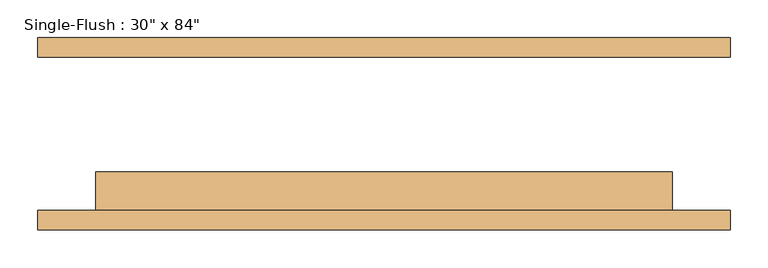
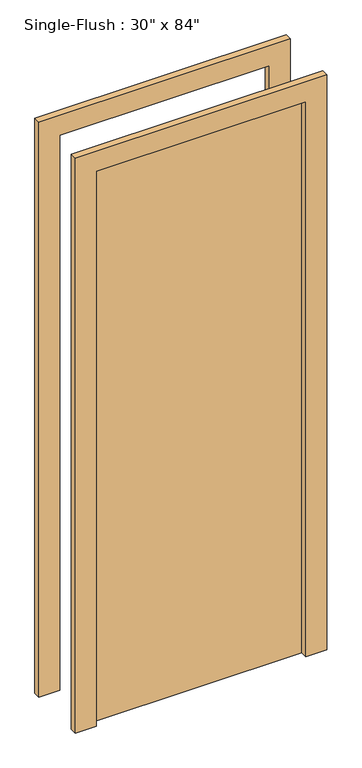
"""IFC4 building model written with IfcOpenShell, lengths in millimetres: door geometry."""

from ifc_helpers import new_model, si_unit, frame, origin, origin_with_axes, place, context, project, spatial, polyline, outline, extrude, source, transform, mapped, element, save


def door_4314e8ec(model_context):
    return source(origin(), model_context, "Body", "SweptSolid", [
        extrude(outline(polyline([(2209.8, -457.2), (0.0, -457.2), (0.0, -381.0), (2133.6, -381.0), (2133.6, 381.0), (0.0, 381.0), (0.0, 457.2), (2209.8, 457.2), (2209.8, -457.2)])), frame((0.0, -127.0, 0.0), z_axis=(0.0, 1.0, 0.0), x_axis=(0.0, 0.0, 1.0)), (0.0, 0.0, 1.0), 25.4),
        extrude(outline(polyline([(2209.8, 457.2), (2209.8, -457.2), (0.0, -457.2), (0.0, -381.0), (2133.6, -381.0), (2133.6, 381.0), (0.0, 381.0), (0.0, 457.2), (2209.8, 457.2)])), frame((0.0, 101.6, 0.0), z_axis=(0.0, 1.0, 0.0), x_axis=(0.0, 0.0, 1.0)), (0.0, 0.0, 1.0), 25.4),
        extrude(outline(polyline([(381.0, -50.8), (381.0, -101.6), (-381.0, -101.6), (-381.0, -50.8), (381.0, -50.8)])), origin_with_axes(), (0.0, 0.0, 1.0), 2133.6),
    ])


if __name__ == "__main__":
    model = new_model("IFC4")
    model_context = context("Model", 3, world=origin())
    ifc_project = project(units=[si_unit("LENGTHUNIT", "METRE", prefix="MILLI")], contexts=[model_context])
    site = spatial("IfcSite", under=ifc_project)
    building = spatial("IfcBuilding", under=site)
    placement = place(None, origin())
    door_shape = door_4314e8ec(model_context)
    element("IfcDoor", 1, ObjectType="Single-Flush : 30\" x 84\"", at=placement, inside=building, context=model_context, shape_type="MappedRepresentation", body=[
        mapped(door_shape, transform((0.0, 0.0, 0.0), x_axis=(1.0, 0.0, 0.0), y_axis=(0.0, 1.0, 0.0), z_axis=(0.0, 0.0, 1.0))),
    ])
    save(model, "model.ifc")

# Revit data of these elements
# Type "Single-Flush : 30\" x 84\""
#   Type Mark = "4"
#   Construction Type Id = "MDOOR"
#   Assembly Code = "C1020"
#   Analytic Construction = "Metal"
#   Thickness = 0' - 2"
#   Heat Transfer Coefficient (U) = 0.651978 BTU/(h·ft²·°F)
#   Height = 7' - 0"
#   Trim Projection Ext = 0' - 1"
#   Trim Projection Int = 0' - 1"
#   Trim Width = 0' - 3"
#   Width = 2' - 6"
#   Define Thermal Properties by = 1
#   Define Thermal Properties by = 1
#   Door Material = Door - Panel
#   Frame Material = Door - Frame
#   Visual Light Transmittance = 0
#   Solar Heat Gain Coefficient = 0
#   Function = (empty or 0)
#   Wall Closure = (empty or 0)
# Element 1 (IfcDoor, "Single-Flush : 30\" x 84\"")
#   Materials on its faces: "Door - Frame", "Door - Panel"
# Materials
#   "Door - Panel": class "Wood", colour RGB 210 159 95, transparency 0, Cost = 0
#   "Door - Frame": colour RGB 118 70 51, transparency 0, Cost = 0
